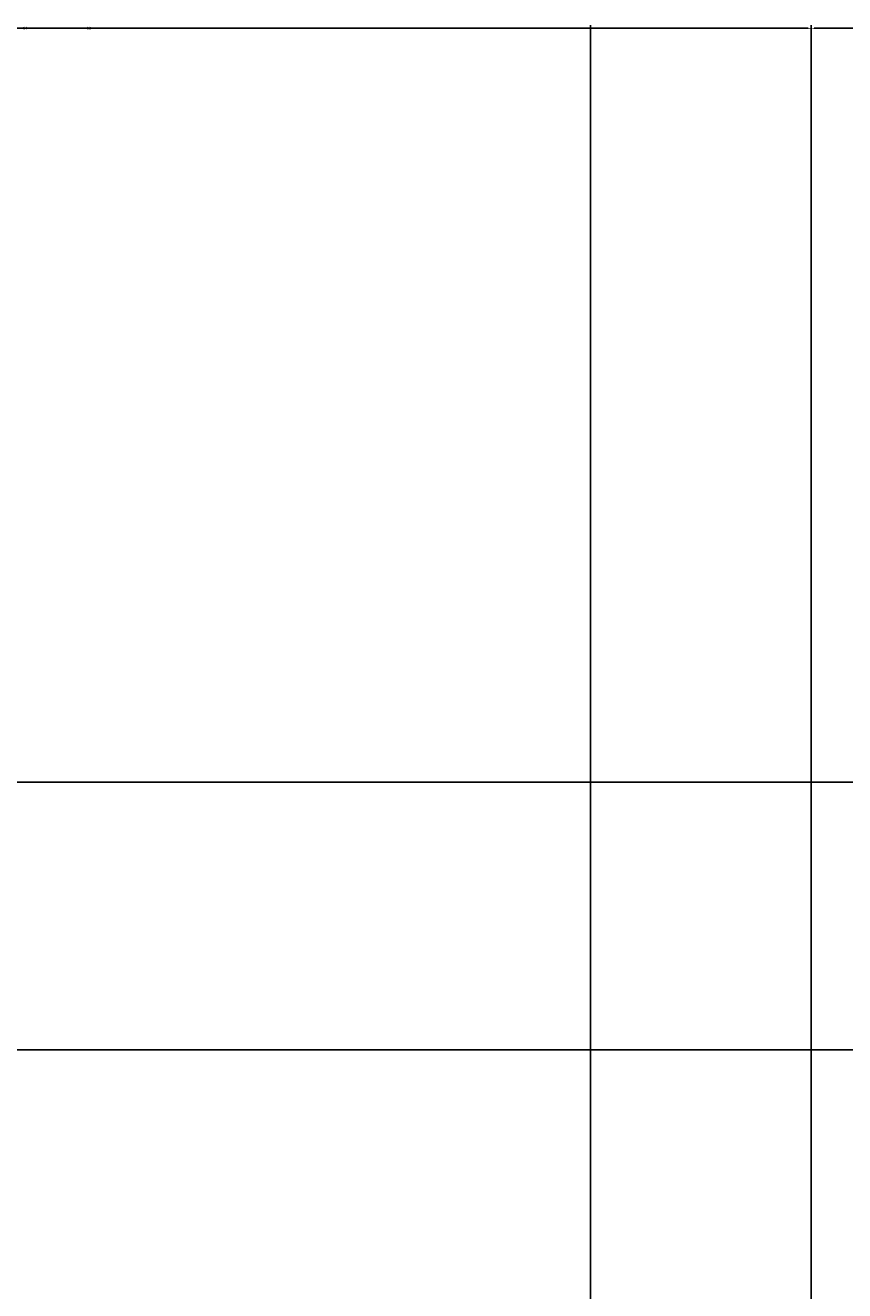
# Model space of a CAD drawing. Units: feet. Extents: x 105 to 1094, y -88 to 588.
# Tile 54 of 59: x 600 to 649, y 513 to 588. Entities that reach past the tile are written whole.
import ezdxf

# ---------------------------------------------------------------- set-up
doc = ezdxf.new("R2010")
doc.units = ezdxf.units.FT
doc.header["$MEASUREMENT"] = 0
doc.layers.add('A-ANNO-DIMS', color=2, linetype='Continuous', lineweight=18)
doc.styles.get("Standard").update_dxf_attribs({"font": 'arial.ttf'})
doc.dimstyles.get("Standard").update_dxf_attribs({"dimtxt": 0.18, "dimasz": 0.18, "dimexe": 0.18, "dimexo": 0.0625, "dimgap": 0.09, "dimtad": 0, "dimtih": 1, "dimtoh": 1, "dimdec": 4, "dimzin": 0, "dimdsep": 46, "dimtxsty": 'Standard', "dimcen": 0.09, "dimadec": 0, "dimazin": 0, "dimtfac": 1, "dimtdec": 4, "dimtofl": 0, "dimtmove": 0, "dimatfit": 3, "dimfxl": 1, "dimtolj": 1, "dimtzin": 0, "dimarcsym": 0})

# ---------------------------------------------------------------- blocks, each defined once
blk = doc.blocks.new('*D21')
at = {"layer": 'A-ANNO-DIMS', "color": 0, "lineweight": -2, "transparency": 16777216}
for p, q in [((849.626, 543.081), (105.458, 543.081)), ((105.638, 542.901), (105.638, 250.263)), ((105.638, -42.739), (105.638, 249.899)), ((849.626, -42.919), (105.458, -42.919))]:
    blk.add_line(p, q, dxfattribs=at)
at = {"layer": 'A-ANNO-DIMS', "color": 0, "transparency": 16777216}
for points in [[(105.608, 542.901), (105.668, 542.901), (105.638, 543.081)], [(105.608, -42.739), (105.668, -42.739), (105.638, -42.919)]]:
    blk.add_solid(points, dxfattribs=at)
at = {"layer": 'Defpoints', "color": 0, "transparency": 16777216}
for p in [(105.638, 543.081), (849.688, 543.081), (849.688, -42.919)]:
    blk.add_point(p, dxfattribs=at)
at = {"layer": 'A-ANNO-DIMS', "color": 0, "transparency": 16777216, "insert": (105.638, 250.081), "char_height": 0.18, "attachment_point": 5}
blk.add_mtext('\\A1;586', dxfattribs=at)
blk = doc.blocks.new('*D26')
at = {"layer": 'A-ANNO-DIMS', "color": 0, "lineweight": -2, "transparency": 16777216}
for p, q in [((552.688, 471.144), (552.688, 588.311)), ((646.688, 471.144), (646.688, 588.311)), ((552.868, 588.131), (599.47, 588.131)), ((646.508, 588.131), (599.907, 588.131))]:
    blk.add_line(p, q, dxfattribs=at)
at = {"layer": 'A-ANNO-DIMS', "color": 0, "transparency": 16777216}
for points in [[(552.868, 588.161), (552.868, 588.101), (552.688, 588.131)], [(646.508, 588.161), (646.508, 588.101), (646.688, 588.131)]]:
    blk.add_solid(points, dxfattribs=at)
at = {"layer": 'Defpoints', "color": 0, "transparency": 16777216}
for p in [(646.688, 588.131), (552.688, 471.081), (646.688, 471.081)]:
    blk.add_point(p, dxfattribs=at)
at = {"layer": 'A-ANNO-DIMS', "color": 0, "transparency": 16777216, "insert": (599.688, 588.131), "char_height": 0.18, "attachment_point": 5}
blk.add_mtext('\\A1;94', dxfattribs=at)
blk = doc.blocks.new('*D30')
at = {"layer": 'A-ANNO-DIMS', "color": 0, "lineweight": -2, "transparency": 16777216}
for p, q in [((349.751, 543.081), (1093.918, 543.081)), ((1093.738, 542.901), (1093.738, 535.263)), ((1093.738, 527.261), (1093.738, 534.899)), ((349.751, 527.081), (1093.918, 527.081))]:
    blk.add_line(p, q, dxfattribs=at)
at = {"layer": 'A-ANNO-DIMS', "color": 0, "transparency": 16777216}
for points in [[(1093.708, 542.901), (1093.768, 542.901), (1093.738, 543.081)], [(1093.708, 527.261), (1093.768, 527.261), (1093.738, 527.081)]]:
    blk.add_solid(points, dxfattribs=at)
at = {"layer": 'Defpoints', "color": 0, "transparency": 16777216}
for p in [(349.688, 543.081), (349.688, 527.081), (1093.738, 527.081)]:
    blk.add_point(p, dxfattribs=at)
at = {"layer": 'A-ANNO-DIMS', "color": 0, "transparency": 16777216, "insert": (1093.738, 535.081), "char_height": 0.18, "attachment_point": 5}
blk.add_mtext('\\A1;16', dxfattribs=at)
blk = doc.blocks.new('*D31')
at = {"layer": 'A-ANNO-DIMS', "color": 0, "lineweight": -2, "transparency": 16777216}
for p, q in [((438.751, 527.081), (1093.918, 527.081)), ((1093.738, 526.901), (1093.738, 499.263)), ((1093.738, 471.261), (1093.738, 498.899)), ((438.751, 471.081), (1093.918, 471.081))]:
    blk.add_line(p, q, dxfattribs=at)
at = {"layer": 'A-ANNO-DIMS', "color": 0, "transparency": 16777216}
for points in [[(1093.708, 526.901), (1093.768, 526.901), (1093.738, 527.081)], [(1093.708, 471.261), (1093.768, 471.261), (1093.738, 471.081)]]:
    blk.add_solid(points, dxfattribs=at)
at = {"layer": 'Defpoints', "color": 0, "transparency": 16777216}
for p in [(438.688, 527.081), (1093.738, 527.081), (438.688, 471.081)]:
    blk.add_point(p, dxfattribs=at)
at = {"layer": 'A-ANNO-DIMS', "color": 0, "transparency": 16777216, "insert": (1093.738, 499.081), "char_height": 0.18, "attachment_point": 5}
blk.add_mtext('\\A1;56', dxfattribs=at)
blk = doc.blocks.new('*D41')
at = {"layer": 'A-ANNO-DIMS', "color": 0, "lineweight": -2, "transparency": 16777216}
for p, q in [((646.688, 441.144), (646.688, 588.311)), ((671.688, 441.144), (671.688, 588.311)), ((646.868, 588.131), (658.967, 588.131)), ((671.508, 588.131), (659.409, 588.131))]:
    blk.add_line(p, q, dxfattribs=at)
at = {"layer": 'A-ANNO-DIMS', "color": 0, "transparency": 16777216}
for points in [[(646.868, 588.161), (646.868, 588.101), (646.688, 588.131)], [(671.508, 588.161), (671.508, 588.101), (671.688, 588.131)]]:
    blk.add_solid(points, dxfattribs=at)
at = {"layer": 'Defpoints', "color": 0, "transparency": 16777216}
for p in [(671.688, 588.131), (646.688, 441.081), (671.688, 441.081)]:
    blk.add_point(p, dxfattribs=at)
at = {"layer": 'A-ANNO-DIMS', "color": 0, "transparency": 16777216, "insert": (659.188, 588.131), "char_height": 0.18, "attachment_point": 5}
blk.add_mtext('\\A1;25', dxfattribs=at)
blk = doc.blocks.new('*D48')
at = {"layer": 'A-ANNO-DIMS', "color": 0, "lineweight": -2, "transparency": 16777216}
for p, q in [((573.483, 441.144), (573.483, 588.311)), ((633.483, 441.144), (633.483, 588.311)), ((573.663, 588.131), (603.263, 588.131)), ((633.303, 588.131), (603.702, 588.131))]:
    blk.add_line(p, q, dxfattribs=at)
at = {"layer": 'A-ANNO-DIMS', "color": 0, "transparency": 16777216}
for points in [[(573.663, 588.161), (573.663, 588.101), (573.483, 588.131)], [(633.303, 588.161), (633.303, 588.101), (633.483, 588.131)]]:
    blk.add_solid(points, dxfattribs=at)
at = {"layer": 'Defpoints', "color": 0, "transparency": 16777216}
for p in [(633.483, 588.131), (573.483, 441.081), (633.483, 441.081)]:
    blk.add_point(p, dxfattribs=at)
at = {"layer": 'A-ANNO-DIMS', "color": 0, "transparency": 16777216, "insert": (603.483, 588.131), "char_height": 0.18, "attachment_point": 5}
blk.add_mtext('\\A1;60', dxfattribs=at)

msp = doc.modelspace()

# ---------------------------------------------------------------- dimensions: what is measured, and where the dimension line sits
at = {"layer": 'A-ANNO-DIMS'}
for base, p1, p2, picture, middle in [((646.6883, 588.1312), (552.6883, 471.0812), (646.6883, 471.0812), '*D26', (599.6883, 588.1312)), ((633.4826, 588.1312), (573.4826, 441.0812), (633.4826, 441.0812), '*D48', (603.4826, 588.1312)), ((671.6883, 588.1312), (646.6883, 441.0812), (671.6883, 441.0812), '*D41', (659.1883, 588.1312))]:
    dim = msp.add_linear_dim(base=base, p1=p1, p2=p2, dimstyle='Standard', override={"dimdec": 0, "dimlfac": 1, "dimrnd": 0, "dimzin": 0, "dimdsep": 46, "dimlunit": 2}, dxfattribs=at)
    dim.commit()
    dim.dimension.update_dxf_attribs({"geometry": picture, "text_midpoint": middle})
for base, p1, p2, picture, middle in [((105.6383, 543.0812), (849.6883, -42.9188), (849.6883, 543.0812), '*D21', (105.6383, 250.0812)), ((1093.7383, 527.0812), (349.6883, 543.0812), (349.6883, 527.0812), '*D30', (1093.7383, 535.0812)), ((1093.7383, 527.0812), (438.6883, 471.0812), (438.6883, 527.0812), '*D31', (1093.7383, 499.0812))]:
    dim = msp.add_linear_dim(base=base, p1=p1, p2=p2, angle=90, dimstyle='Standard', override={"dimdec": 0, "dimlfac": 1, "dimrnd": 0, "dimzin": 0, "dimdsep": 46, "dimlunit": 2}, dxfattribs=at)
    dim.commit()
    dim.dimension.update_dxf_attribs({"geometry": picture, "text_midpoint": middle})

doc.saveas('drawing.dxf')
